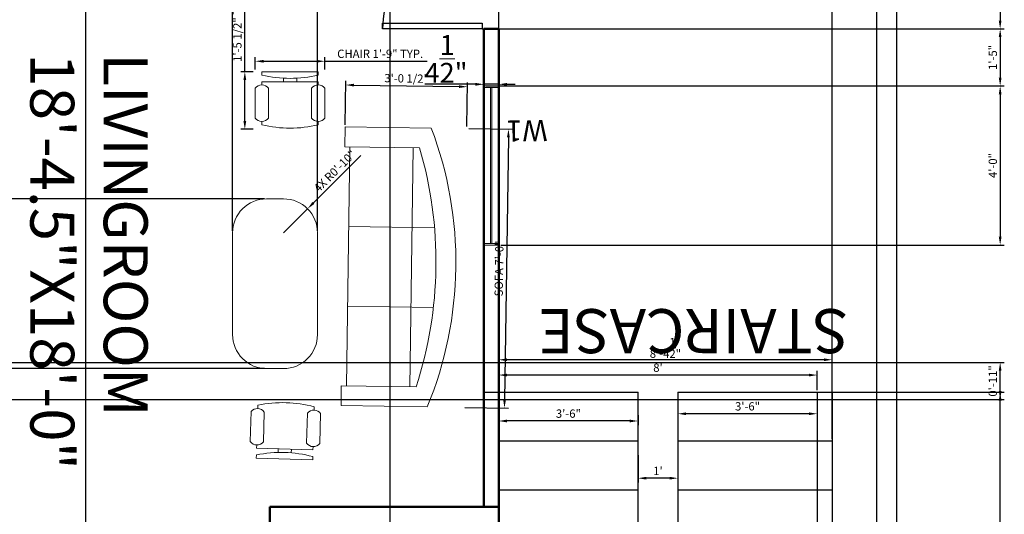
# Model space of a CAD drawing. Units: inches. Extents: x 1989 to 2637, y 1032 to 1611.
# Tile 4 of 5: x 2340 to 2637, y 1274 to 1423. Entities that reach past the tile are written whole.
import ezdxf

# ---------------------------------------------------------------- set-up
doc = ezdxf.new("R2010")
doc.units = ezdxf.units.IN
for name, color, linetype, lineweight in [('A-ANNO-TEXT', 1, 'Continuous', 18), ('A-AREA-IDEN', 1, 'Continuous', 25), ('C-PROP', 7, 'Continuous', 25), ('DIMENSIONS', 7, 'Continuous', 18), ('doors', 5, 'Continuous', 25), ('furniture', 8, 'Continuous', 18), ('stair case', 6, 'Continuous', 25), ('walls', 7, 'Continuous', 50), ('windows', 3, 'Continuous', 18)]:
    doc.layers.add(name, color=color, linetype=linetype, lineweight=lineweight)
doc.styles.get("Standard").update_dxf_attribs({"font": 'arial.ttf'})
doc.dimstyles.new('ISO-25', dxfattribs={"dimtxt": 2.5, "dimasz": 2.5, "dimexe": 1.25, "dimexo": 0.625, "dimtad": 1, "dimlunit": 4, "dimtxsty": 'Standard', "dimcen": 2.5, "dimadec": 0, "dimazin": 0, "dimtfac": 1, "dimtmove": 0, "dimatfit": 3, "dimfxl": 1, "dimarcsym": 0})

# ---------------------------------------------------------------- blocks, each defined once
blk = doc.blocks.new('*U2')
for p, q in [((0, 0), (0, -5)), ((30, 0), (30, -5))]:
    blk.add_line(p, q)
blk.add_lwpolyline([(0, 0), (0, 30), (1.75, 30), (1.75, 0)], close=True)
blk.add_arc((0, 0), 30, 0, 90)
blk = doc.blocks.new('Sofa - Roundback 7 ft.')
for p, q in [((-12.00002, -32.4421), (-12.00003, -6.5971)), ((11.99997, -32.4421), (11.99998, -6.5971)), ((-36.000027, -34), (-36.000027, -11.4696)), ((35.99998, -34), (35.99998, -11.4696)), ((-35.999844, -13.3819), (35.9998, -13.3819)), ((-36.000027, -32.4421), (35.99998, -32.4421))]:
    blk.add_line(p, q)
for points in [[(-36.000027, -34), (-42.000027, -34), (-42.000027, -8)], [(41.99998, -8), (41.99998, -34), (35.99998, -34)]]:
    blk.add_lwpolyline(points)
for centre, radius, start, end in [((0, -114.25), 114.25, 68.43141, 111.5686), ((-0.00001, -127.1968), 121.1968, 72.72033, 107.2797)]:
    blk.add_arc(centre, radius, start, end)
blk = doc.blocks.new('Chair - Desk')
for p, q in [((-8.5, 0), (-8.5, -1)), ((-8.5, 0), (8.5, 0)), ((8.5, 0), (8.5, -1)), ((-2, -3), (-2, -1.9355)), ((2, -1.9576), (2, -3)), ((-10.5, -5), (-10.5, -14)), ((-8.5, -3), (-8.5, -4)), ((-8.5, -3), (8.5, -3)), ((-6.5, -14), (-6.5, -5)), ((6.5, -5), (6.5, -14)), ((8.5, -3), (8.5, -4)), ((10.5, -14), (10.5, -5)), ((-8.5, -15), (-8.5, -16)), ((8.5, -15), (8.5, -16))]:
    blk.add_line(p, q)
for centre, radius, start, end in [((0, 34.625), 36.625, 256.5803, 283.4197), ((-8.5, -6.5), 2.5, 36.8699, 143.1301), ((8.5, -6.5), 2.5, 36.8699, 143.1301), ((-8.5, -12.5), 2.5, 216.8699, 323.1301), ((8.5, -12.5), 2.5, 216.8699, 323.1301), ((0, 19.625), 36.625, 256.5803, 283.4197)]:
    blk.add_arc(centre, radius, start, end)
blk = doc.blocks.new('*D13')
at = {"layer": 'Defpoints', "color": 0, "transparency": 16777216}
for p in [(2484.5, 1432.53), (2484.5, 1402.72), (2598.5, 1403.71)]:
    blk.add_point(p, dxfattribs=at)
at = {"layer": 'DIMENSIONS', "color": 0, "lineweight": -2, "transparency": 16777216}
for p, q in [((2484.5, 1403.34), (2484.5, 1433.78)), ((2598.5, 1404.33), (2598.5, 1433.78)), ((2596, 1432.53), (2487, 1432.53))]:
    blk.add_line(p, q, dxfattribs=at)
at = {"layer": 'DIMENSIONS', "color": 0, "transparency": 16777216}
for points in [[(2487, 1432.95), (2487, 1432.12), (2484.5, 1432.53)], [(2596, 1432.95), (2596, 1432.12), (2598.5, 1432.53)]]:
    blk.add_solid(points, dxfattribs=at)
at = {"layer": 'DIMENSIONS', "color": 0, "transparency": 16777216, "insert": (2541.5, 1436.22), "char_height": 6, "attachment_point": 5}
blk.add_mtext('9\'-6"', dxfattribs=at)
blk = doc.blocks.new('*D15')
at = {"layer": 'Defpoints', "color": 0, "transparency": 16777216}
for p in [(2480, 1411.38), (2484.5, 1411.38), (2480, 1403.71)]:
    blk.add_point(p, dxfattribs=at)
at = {"layer": 'DIMENSIONS', "color": 0, "lineweight": -2, "transparency": 16777216}
for p, q in [((2480, 1410.76), (2480, 1402.46)), ((2484.5, 1410.76), (2484.5, 1402.46)), ((2477.5, 1403.71), (2462.23, 1403.71)), ((2484.5, 1403.71), (2480, 1403.71)), ((2487, 1403.71), (2489.5, 1403.71))]:
    blk.add_line(p, q, dxfattribs=at)
at = {"layer": 'DIMENSIONS', "color": 0, "transparency": 16777216}
for points in [[(2477.5, 1404.13), (2477.5, 1403.3), (2480, 1403.71)], [(2487, 1404.13), (2487, 1403.3), (2484.5, 1403.71)]]:
    blk.add_solid(points, dxfattribs=at)
at = {"layer": 'DIMENSIONS', "color": 0, "transparency": 16777216, "insert": (2468.62, 1411.36), "char_height": 6, "attachment_point": 5}
blk.add_mtext('4{\\H1x;\\S1/2;}"', dxfattribs=at)
blk = doc.blocks.new('*D17')
at = {"layer": 'Defpoints', "color": 0, "transparency": 16777216}
for p in [(2538.5, 1310.92), (2580.5, 1310.92), (2538.5, 1304.46)]:
    blk.add_point(p, dxfattribs=at)
at = {"layer": 'DIMENSIONS', "color": 0, "lineweight": -2, "transparency": 16777216}
for p, q in [((2538.5, 1310.3), (2538.5, 1303.21)), ((2580.5, 1310.3), (2580.5, 1303.21)), ((2578, 1304.46), (2541, 1304.46))]:
    blk.add_line(p, q, dxfattribs=at)
at = {"layer": 'DIMENSIONS', "color": 0, "transparency": 16777216}
for points in [[(2541, 1304.88), (2541, 1304.05), (2538.5, 1304.46)], [(2578, 1304.88), (2578, 1304.05), (2580.5, 1304.46)]]:
    blk.add_solid(points, dxfattribs=at)
at = {"layer": 'DIMENSIONS', "color": 0, "transparency": 16777216, "insert": (2559.5, 1306.37), "char_height": 2.5, "attachment_point": 5}
blk.add_mtext('3\'-6"', dxfattribs=at)
blk = doc.blocks.new('*D18')
at = {"layer": 'Defpoints', "color": 0, "transparency": 16777216}
for p in [(2526.5, 1292.57), (2538.5, 1292.57), (2526.5, 1285.04)]:
    blk.add_point(p, dxfattribs=at)
at = {"layer": 'DIMENSIONS', "color": 0, "lineweight": -2, "transparency": 16777216}
for p, q in [((2526.5, 1291.94), (2526.5, 1283.79)), ((2538.5, 1291.94), (2538.5, 1283.79)), ((2536, 1285.04), (2529, 1285.04))]:
    blk.add_line(p, q, dxfattribs=at)
at = {"layer": 'DIMENSIONS', "color": 0, "transparency": 16777216}
for points in [[(2529, 1285.46), (2529, 1284.63), (2526.5, 1285.04)], [(2536, 1285.46), (2536, 1284.63), (2538.5, 1285.04)]]:
    blk.add_solid(points, dxfattribs=at)
at = {"layer": 'DIMENSIONS', "color": 0, "transparency": 16777216, "insert": (2532.5, 1286.92), "char_height": 2.5, "attachment_point": 5}
blk.add_mtext("1'", dxfattribs=at)
blk = doc.blocks.new('*D19')
at = {"layer": 'Defpoints', "color": 0, "transparency": 16777216}
for p in [(2484.5, 1304.71), (2526.5, 1304.71), (2484.5, 1302.28)]:
    blk.add_point(p, dxfattribs=at)
at = {"layer": 'DIMENSIONS', "color": 0, "lineweight": -2, "transparency": 16777216}
for p, q in [((2484.5, 1304.08), (2484.5, 1301.03)), ((2526.5, 1304.08), (2526.5, 1301.03)), ((2524, 1302.28), (2487, 1302.28))]:
    blk.add_line(p, q, dxfattribs=at)
at = {"layer": 'DIMENSIONS', "color": 0, "transparency": 16777216}
for points in [[(2487, 1302.7), (2487, 1301.86), (2484.5, 1302.28)], [(2524, 1302.7), (2524, 1301.86), (2526.5, 1302.28)]]:
    blk.add_solid(points, dxfattribs=at)
at = {"layer": 'DIMENSIONS', "color": 0, "transparency": 16777216, "insert": (2505.5, 1304.18), "char_height": 2.5, "attachment_point": 5}
blk.add_mtext('3\'-6"', dxfattribs=at)
blk = doc.blocks.new('*D20')
at = {"layer": 'Defpoints', "color": 0, "transparency": 16777216}
for p in [(2484.5, 1316.12), (2484.5, 1310.92), (2580.5, 1310.92)]:
    blk.add_point(p, dxfattribs=at)
at = {"layer": 'DIMENSIONS', "color": 0, "lineweight": -2, "transparency": 16777216}
for p, q in [((2484.5, 1311.55), (2484.5, 1317.37)), ((2578, 1316.12), (2487, 1316.12)), ((2580.5, 1311.55), (2580.5, 1317.37))]:
    blk.add_line(p, q, dxfattribs=at)
at = {"layer": 'DIMENSIONS', "color": 0, "transparency": 16777216}
for points in [[(2487, 1316.53), (2487, 1315.7), (2484.5, 1316.12)], [(2578, 1316.53), (2578, 1315.7), (2580.5, 1316.12)]]:
    blk.add_solid(points, dxfattribs=at)
at = {"layer": 'DIMENSIONS', "color": 0, "transparency": 16777216, "insert": (2532.5, 1318.02), "char_height": 2.5, "attachment_point": 5}
blk.add_mtext("8'", dxfattribs=at)
blk = doc.blocks.new('*D21')
at = {"layer": 'Defpoints', "color": 0, "transparency": 16777216}
for p in [(2484.5, 1320.73), (2484.5, 1296.25), (2585, 1296.25)]:
    blk.add_point(p, dxfattribs=at)
at = {"layer": 'DIMENSIONS', "color": 0, "lineweight": -2, "transparency": 16777216}
for p, q in [((2484.5, 1296.88), (2484.5, 1321.98)), ((2582.5, 1320.73), (2487, 1320.73)), ((2585, 1296.88), (2585, 1321.98))]:
    blk.add_line(p, q, dxfattribs=at)
at = {"layer": 'DIMENSIONS', "color": 0, "transparency": 16777216}
for points in [[(2487, 1321.15), (2487, 1320.31), (2484.5, 1320.73)], [(2582.5, 1321.15), (2582.5, 1320.31), (2585, 1320.73)]]:
    blk.add_solid(points, dxfattribs=at)
at = {"layer": 'DIMENSIONS', "color": 0, "transparency": 16777216, "insert": (2534.75, 1324.3), "char_height": 2.5, "attachment_point": 5}
blk.add_mtext('8\'-4{\\H1x;\\S1/2;}"', dxfattribs=at)
blk = doc.blocks.new('*D28')
at = {"layer": 'Defpoints', "color": 0, "transparency": 16777216}
for p in [(2432.12, 1410.66), (2411.12, 1407.51), (2432.12, 1407.51)]:
    blk.add_point(p, dxfattribs=at)
at = {"layer": 'DIMENSIONS', "color": 0, "lineweight": -2, "transparency": 16777216}
for p, q in [((2411.12, 1408.13), (2411.12, 1411.91)), ((2413.62, 1410.66), (2429.62, 1410.66)), ((2432.12, 1408.13), (2432.12, 1411.91)), ((2432.12, 1410.66), (2462.92, 1410.66))]:
    blk.add_line(p, q, dxfattribs=at)
at = {"layer": 'DIMENSIONS', "color": 0, "transparency": 16777216}
for points in [[(2413.62, 1411.07), (2413.62, 1410.24), (2411.12, 1410.66)], [(2429.62, 1411.07), (2429.62, 1410.24), (2432.12, 1410.66)]]:
    blk.add_solid(points, dxfattribs=at)
at = {"layer": 'DIMENSIONS', "color": 0, "transparency": 16777216, "insert": (2448.77, 1412.58), "char_height": 2.5, "attachment_point": 5}
blk.add_mtext('CHAIR 1\'-9" TYP.', dxfattribs=at)
blk = doc.blocks.new('*D29')
at = {"layer": 'Defpoints', "color": 0, "transparency": 16777216}
for p in [(2407.97, 1407.51), (2411.12, 1407.51), (2411.12, 1390.17)]:
    blk.add_point(p, dxfattribs=at)
at = {"layer": 'DIMENSIONS', "color": 0, "lineweight": -2, "transparency": 16777216}
for p, q in [((2407.97, 1407.51), (2407.97, 1432.09)), ((2410.49, 1407.51), (2406.72, 1407.51)), ((2407.97, 1392.67), (2407.97, 1405.01)), ((2410.49, 1390.17), (2406.72, 1390.17))]:
    blk.add_line(p, q, dxfattribs=at)
at = {"layer": 'DIMENSIONS', "color": 0, "transparency": 16777216}
for points in [[(2407.55, 1405.01), (2408.39, 1405.01), (2407.97, 1407.51)], [(2407.55, 1392.67), (2408.39, 1392.67), (2407.97, 1390.17)]]:
    blk.add_solid(points, dxfattribs=at)
at = {"layer": 'DIMENSIONS', "color": 0, "transparency": 16777216, "insert": (2406.05, 1421.05), "char_height": 2.5, "attachment_point": 5, "rotation": 90}
blk.add_mtext('1\'-5 1/2" TYP.', dxfattribs=at)
blk = doc.blocks.new('*D36')
at = {"layer": 'Defpoints', "color": 0, "transparency": 16777216}
for p in [(2474.85, 1390.38), (2473.63, 1306.39), (2486.23, 1306.2)]:
    blk.add_point(p, dxfattribs=at)
at = {"layer": 'DIMENSIONS', "color": 0, "lineweight": -2, "transparency": 16777216}
for p, q in [((2475.47, 1390.37), (2488.7, 1390.18)), ((2487.41, 1387.7), (2486.27, 1308.7)), ((2474.26, 1306.38), (2487.48, 1306.19))]:
    blk.add_line(p, q, dxfattribs=at)
at = {"layer": 'DIMENSIONS', "color": 0, "transparency": 16777216}
for points in [[(2486.99, 1387.7), (2487.83, 1387.69), (2487.45, 1390.2)], [(2485.85, 1308.71), (2486.68, 1308.7), (2486.23, 1306.2)]]:
    blk.add_solid(points, dxfattribs=at)
at = {"layer": 'DIMENSIONS', "color": 0, "transparency": 16777216, "insert": (2484.92, 1348.23), "char_height": 2.5, "attachment_point": 5, "rotation": 89.1706}
blk.add_mtext('SOFA 7\'-0"', dxfattribs=at)
blk = doc.blocks.new('*D37')
at = {"layer": 'Defpoints', "color": 0, "transparency": 16777216}
for p in [(2475.03, 1402.98), (2438.19, 1390.91), (2474.85, 1390.38)]:
    blk.add_point(p, dxfattribs=at)
at = {"layer": 'DIMENSIONS', "color": 0, "lineweight": -2, "transparency": 16777216}
for p, q in [((2438.2, 1391.53), (2438.39, 1404.76)), ((2474.86, 1391), (2475.05, 1404.23)), ((2440.87, 1403.47), (2472.53, 1403.01))]:
    blk.add_line(p, q, dxfattribs=at)
at = {"layer": 'DIMENSIONS', "color": 0, "transparency": 16777216}
for points in [[(2440.87, 1403.89), (2440.86, 1403.05), (2438.37, 1403.51)], [(2472.54, 1403.43), (2472.53, 1402.6), (2475.03, 1402.98)]]:
    blk.add_solid(points, dxfattribs=at)
at = {"layer": 'DIMENSIONS', "color": 0, "transparency": 16777216, "insert": (2456.73, 1405.16), "char_height": 2.5, "attachment_point": 5, "rotation": 359.1706}
blk.add_mtext('3\'-0 1/2"', dxfattribs=at)
blk = doc.blocks.new('*D40')
at = {"layer": 'Defpoints', "color": 0, "transparency": 16777216}
for p in [(2585, 1576.07), (2082.5, 1496.92), (2585, 1310.92)]:
    blk.add_point(p, dxfattribs=at)
at = {"layer": 'DIMENSIONS', "color": 0, "lineweight": -2, "transparency": 16777216}
for p, q in [((2082.5, 1497.55), (2082.5, 1577.32)), ((2085, 1576.07), (2582.5, 1576.07)), ((2585, 1311.55), (2585, 1577.32))]:
    blk.add_line(p, q, dxfattribs=at)
at = {"layer": 'DIMENSIONS', "color": 0, "transparency": 16777216}
for points in [[(2085, 1576.49), (2085, 1575.65), (2082.5, 1576.07)], [(2582.5, 1576.49), (2582.5, 1575.65), (2585, 1576.07)]]:
    blk.add_solid(points, dxfattribs=at)
at = {"layer": 'DIMENSIONS', "color": 0, "transparency": 16777216, "insert": (2333.75, 1577.99), "char_height": 2.5, "attachment_point": 5}
blk.add_mtext('41\'-10 1/2"', dxfattribs=at)
blk = doc.blocks.new('*D42')
at = {"layer": 'Defpoints', "color": 0, "transparency": 16777216}
for p in [(2484.5, 1480.42), (2484.5, 1420.42), (2635.65, 1420.42)]:
    blk.add_point(p, dxfattribs=at)
at = {"layer": 'DIMENSIONS', "color": 0, "lineweight": -2, "transparency": 16777216}
for p, q in [((2485.12, 1480.42), (2636.9, 1480.42)), ((2635.65, 1477.92), (2635.65, 1422.92)), ((2485.12, 1420.42), (2636.9, 1420.42))]:
    blk.add_line(p, q, dxfattribs=at)
at = {"layer": 'DIMENSIONS', "color": 0, "transparency": 16777216}
for points in [[(2635.23, 1477.92), (2636.06, 1477.92), (2635.65, 1480.42)], [(2635.23, 1422.92), (2636.06, 1422.92), (2635.65, 1420.42)]]:
    blk.add_solid(points, dxfattribs=at)
at = {"layer": 'DIMENSIONS', "color": 0, "transparency": 16777216, "insert": (2633.75, 1450.42), "char_height": 2.5, "attachment_point": 5, "rotation": 90}
blk.add_mtext('5\'-0"', dxfattribs=at)
blk = doc.blocks.new('*D46')
at = {"layer": 'Defpoints', "color": 0, "transparency": 16777216}
for p in [(2484.5, 1403.22), (2484.5, 1355.27), (2635.65, 1355.27)]:
    blk.add_point(p, dxfattribs=at)
at = {"layer": 'DIMENSIONS', "color": 0, "lineweight": -2, "transparency": 16777216}
for p, q in [((2485.12, 1403.22), (2636.9, 1403.22)), ((2635.65, 1400.72), (2635.65, 1357.77)), ((2485.12, 1355.27), (2636.9, 1355.27))]:
    blk.add_line(p, q, dxfattribs=at)
at = {"layer": 'DIMENSIONS', "color": 0, "transparency": 16777216}
for points in [[(2635.23, 1400.72), (2636.06, 1400.72), (2635.65, 1403.22)], [(2635.23, 1357.77), (2636.06, 1357.77), (2635.65, 1355.27)]]:
    blk.add_solid(points, dxfattribs=at)
at = {"layer": 'DIMENSIONS', "color": 0, "transparency": 16777216, "insert": (2633.75, 1379.24), "char_height": 2.5, "attachment_point": 5, "rotation": 90}
blk.add_mtext('4\'-0"', dxfattribs=at)
blk = doc.blocks.new('*D47')
at = {"layer": 'Defpoints', "color": 0, "transparency": 16777216}
for p in [(2580.5, 1310.92), (2635.65, 1310.92), (2585, 1178.92)]:
    blk.add_point(p, dxfattribs=at)
at = {"layer": 'DIMENSIONS', "color": 0, "lineweight": -2, "transparency": 16777216}
for p, q in [((2581.12, 1310.92), (2636.9, 1310.92)), ((2635.65, 1181.42), (2635.65, 1308.42)), ((2585.62, 1178.92), (2636.9, 1178.92))]:
    blk.add_line(p, q, dxfattribs=at)
at = {"layer": 'DIMENSIONS', "color": 0, "transparency": 16777216}
for points in [[(2635.23, 1308.42), (2636.06, 1308.42), (2635.65, 1310.92)], [(2635.23, 1181.42), (2636.06, 1181.42), (2635.65, 1178.92)]]:
    blk.add_solid(points, dxfattribs=at)
at = {"layer": 'DIMENSIONS', "color": 0, "transparency": 16777216, "insert": (2633.75, 1244.92), "char_height": 2.5, "attachment_point": 5, "rotation": 90}
blk.add_mtext('11\'-0"', dxfattribs=at)
blk = doc.blocks.new('*D54')
at = {"layer": 'Defpoints', "color": 0, "transparency": 16777216}
for p in [(2429.87, 1576.07), (2404.3, 1358.98), (2429.87, 1358.98)]:
    blk.add_point(p, dxfattribs=at)
at = {"layer": 'DIMENSIONS', "color": 0, "lineweight": -2, "transparency": 16777216}
for p, q in [((2404.3, 1359.6), (2404.3, 1577.32)), ((2406.8, 1576.07), (2427.37, 1576.07)), ((2429.87, 1359.6), (2429.87, 1577.32))]:
    blk.add_line(p, q, dxfattribs=at)
at = {"layer": 'DIMENSIONS', "color": 0, "transparency": 16777216}
for points in [[(2406.8, 1576.49), (2406.8, 1575.65), (2404.3, 1576.07)], [(2427.37, 1576.49), (2427.37, 1575.65), (2429.87, 1576.07)]]:
    blk.add_solid(points, dxfattribs=at)
at = {"layer": 'DIMENSIONS', "color": 0, "transparency": 16777216, "insert": (2417.08, 1577.99), "char_height": 2.5, "attachment_point": 5}
blk.add_mtext('2\'-1 1/2"', dxfattribs=at)
blk = doc.blocks.new('*D55')
at = {"layer": 'Defpoints', "color": 0, "transparency": 16777216}
for p in [(2414.53, 1369.21), (2033.35, 1318.07), (2414.53, 1318.07)]:
    blk.add_point(p, dxfattribs=at)
at = {"layer": 'DIMENSIONS', "color": 0, "lineweight": -2, "transparency": 16777216}
for p, q in [((2413.9, 1369.21), (2032.1, 1369.21)), ((2033.35, 1366.71), (2033.35, 1320.57)), ((2413.9, 1318.07), (2032.1, 1318.07))]:
    blk.add_line(p, q, dxfattribs=at)
at = {"layer": 'DIMENSIONS', "color": 0, "transparency": 16777216}
for points in [[(2032.93, 1366.71), (2033.76, 1366.71), (2033.35, 1369.21)], [(2032.93, 1320.57), (2033.76, 1320.57), (2033.35, 1318.07)]]:
    blk.add_solid(points, dxfattribs=at)
at = {"layer": 'DIMENSIONS', "color": 0, "transparency": 16777216, "insert": (2031.45, 1343.64), "char_height": 2.5, "attachment_point": 5, "rotation": 90}
blk.add_mtext('4\'-3"', dxfattribs=at)
blk = doc.blocks.new('*D58')
at = {"layer": 'Defpoints', "color": 0, "transparency": 16777216}
for p in [(2480, 1420.42), (2480, 1403.22), (2635.65, 1403.22)]:
    blk.add_point(p, dxfattribs=at)
at = {"layer": 'DIMENSIONS', "color": 0, "lineweight": -2, "transparency": 16777216}
for p, q in [((2480.62, 1420.42), (2636.9, 1420.42)), ((2635.65, 1417.92), (2635.65, 1405.72)), ((2480.62, 1403.22), (2636.9, 1403.22))]:
    blk.add_line(p, q, dxfattribs=at)
at = {"layer": 'DIMENSIONS', "color": 0, "transparency": 16777216}
for points in [[(2635.23, 1417.92), (2636.06, 1417.92), (2635.65, 1420.42)], [(2635.23, 1405.72), (2636.06, 1405.72), (2635.65, 1403.22)]]:
    blk.add_solid(points, dxfattribs=at)
at = {"layer": 'DIMENSIONS', "color": 0, "transparency": 16777216, "insert": (2633.75, 1411.82), "char_height": 2.5, "attachment_point": 5, "rotation": 90}
blk.add_mtext('1\'-5"', dxfattribs=at)
blk = doc.blocks.new('*D60')
at = {"layer": 'Defpoints', "color": 0, "transparency": 16777216}
for p in [(2451.78, 1576.07), (2360, 1087.42), (2451.78, 1087.42)]:
    blk.add_point(p, dxfattribs=at)
at = {"layer": 'DIMENSIONS', "color": 0, "lineweight": -2, "transparency": 16777216}
for p, q in [((2360, 1088.05), (2360, 1577.32)), ((2362.5, 1576.07), (2449.28, 1576.07)), ((2451.78, 1088.05), (2451.78, 1577.32))]:
    blk.add_line(p, q, dxfattribs=at)
at = {"layer": 'DIMENSIONS', "color": 0, "transparency": 16777216}
for points in [[(2362.5, 1576.49), (2362.5, 1575.65), (2360, 1576.07)], [(2449.28, 1576.49), (2449.28, 1575.65), (2451.78, 1576.07)]]:
    blk.add_solid(points, dxfattribs=at)
at = {"layer": 'DIMENSIONS', "color": 0, "transparency": 16777216, "insert": (2405.89, 1577.97), "char_height": 2.5, "attachment_point": 5}
blk.add_mtext('7\'-8"', dxfattribs=at)
blk = doc.blocks.new('*D63')
at = {"layer": 'Defpoints', "color": 0, "transparency": 16777216}
for p in [(2087, 1319.92), (2635.65, 1319.92), (2087, 1308.78)]:
    blk.add_point(p, dxfattribs=at)
at = {"layer": 'DIMENSIONS', "color": 0, "lineweight": -2, "transparency": 16777216}
for p, q in [((2087.62, 1319.92), (2636.9, 1319.92)), ((2635.65, 1311.28), (2635.65, 1317.42)), ((2087.62, 1308.78), (2636.9, 1308.78))]:
    blk.add_line(p, q, dxfattribs=at)
at = {"layer": 'DIMENSIONS', "color": 0, "transparency": 16777216}
for points in [[(2635.23, 1317.42), (2636.06, 1317.42), (2635.65, 1319.92)], [(2635.23, 1311.28), (2636.06, 1311.28), (2635.65, 1308.78)]]:
    blk.add_solid(points, dxfattribs=at)
at = {"layer": 'DIMENSIONS', "color": 0, "transparency": 16777216, "insert": (2633.75, 1314.35), "char_height": 2.5, "attachment_point": 5, "rotation": 90}
blk.add_mtext('0\'-11"', dxfattribs=at)
blk = doc.blocks.new('*D66')
at = {"layer": 'Defpoints', "color": 0, "transparency": 16777216}
for p in [(2426.87, 1366.21), (2419.64, 1358.98)]:
    blk.add_point(p, dxfattribs=at)
at = {"layer": 'DIMENSIONS', "color": 0, "lineweight": -2, "transparency": 16777216}
for p, q in [((2442.93, 1382.27), (2428.64, 1367.98)), ((2419.64, 1358.98), (2426.87, 1366.21))]:
    blk.add_line(p, q, dxfattribs=at)
at = {"layer": 'DIMENSIONS', "color": 0, "transparency": 16777216}
blk.add_solid([(2428.35, 1368.27), (2428.94, 1367.68), (2426.87, 1366.21)], dxfattribs=at)
at = {"layer": 'DIMENSIONS', "color": 0, "transparency": 16777216, "insert": (2435.32, 1377.35), "char_height": 2.5, "attachment_point": 5, "rotation": 45.002}
blk.add_mtext('4X R0\'-10"', dxfattribs=at)

msp = doc.modelspace()

# ---------------------------------------------------------------- linework, layer by layer
at = {"layer": 'C-PROP'}
for p, q in [((2604.498, 1064.921), (2604.498, 1544.921)), ((2598.498, 1070.921), (2598.498, 1538.921))]:
    msp.add_line(p, q, dxfattribs=at)
at = {"layer": 'furniture'}
msp.add_lwpolyline([(2429.87, 1358.979, 0.4142136), (2419.641, 1369.207), (2414.527, 1369.207, 0.4142136), (2404.299, 1358.979), (2404.299, 1328.294, 0.4142136), (2414.527, 1318.065), (2419.641, 1318.065, 0.4142136), (2429.87, 1328.294)], format="xyb", close=True, dxfattribs=at)
at = {"layer": 'stair case'}
for p, q in [((2479.998, 1310.921), (2526.498, 1310.921)), ((2479.998, 1310.921), (2526.498, 1310.921)), ((2484.498, 1070.921), (2484.498, 1310.921)), ((2526.498, 1178.921), (2526.498, 1310.921)), ((2538.498, 1310.921), (2538.498, 1178.921)), ((2538.498, 1310.921), (2584.998, 1310.921)), ((2538.498, 1310.921), (2584.998, 1310.921)), ((2580.498, 1310.921), (2580.498, 1070.921)), ((2584.998, 1310.921), (2584.998, 1070.921)), ((2484.498, 1296.254), (2526.498, 1296.254)), ((2538.498, 1296.254), (2584.998, 1296.254)), ((2484.498, 1281.588), (2526.498, 1281.588)), ((2538.498, 1281.588), (2584.998, 1281.588))]:
    msp.add_line(p, q, dxfattribs=at)
at = {"layer": 'walls'}
for p, q in [((2479.998, 1420.421), (2479.998, 1276.421)), ((2479.998, 1420.421), (2484.498, 1420.421)), ((2484.498, 1420.421), (2484.498, 1276.421)), ((2484.498, 1310.921), (2484.498, 1070.921)), ((2415.498, 1276.421), (2484.498, 1276.421)), ((2415.498, 1276.421), (2415.498, 1259.921))]:
    msp.add_line(p, q, dxfattribs=at)
at = {"layer": 'windows'}
for p, q in [((2479.998, 1355.269), (2479.998, 1403.219)), ((2479.998, 1403.219), (2484.498, 1403.219)), ((2479.998, 1402.719), (2484.498, 1402.719)), ((2482.048, 1402.719), (2482.048, 1355.769)), ((2482.448, 1402.719), (2482.448, 1355.769)), ((2484.498, 1403.219), (2484.498, 1355.269)), ((2484.498, 1355.769), (2479.998, 1355.769)), ((2484.498, 1355.269), (2479.998, 1355.269))]:
    msp.add_line(p, q, dxfattribs=at)

# ---------------------------------------------------------------- block references
at = {"layer": 'doors', "rotation": 89.99999999999999}
msp.add_blockref('*U2', (2479.498, 1420.421), dxfattribs=at)
at = {"layer": 'furniture'}
msp.add_blockref('Chair - Desk', (2421.619, 1407.508), dxfattribs=at)
at = {"layer": 'furniture', "rotation": 269.1705843501265}
msp.add_blockref('Sofa - Roundback 7 ft.', (2471.575, 1348.421), dxfattribs=at)
at = {"layer": 'furniture', "xscale": -1, "rotation": 178.3411687002522}
msp.add_blockref('Chair - Desk', (2419.929, 1290.805), dxfattribs=at)

# ---------------------------------------------------------------- texts
at = {"layer": 'A-ANNO-TEXT', "insert": (2499.262, 1386.594), "char_height": 6.3507, "attachment_point": 1, "rotation": 180.67334}
msp.add_mtext_dynamic_manual_height_columns('W1', width=5.29651, gutter_width=31.753, heights=[0], dxfattribs=at)
at = {"layer": 'A-AREA-IDEN', "attachment_point": 1}
for s, insert, char_height, rotation in [('LIVINGROOM\\P18\'-4.5"X18\'-0"', (2378.703, 1413.037), 13.26964, 270), ('STAIRCASE', (2589.929, 1322.707), 13.2696, 180)]:
    msp.add_mtext_dynamic_manual_height_columns(s, width=13.72319, gutter_width=66.348, heights=[0], dxfattribs=dict(at, insert=insert, char_height=char_height, rotation=rotation))

# ---------------------------------------------------------------- dimensions: what is measured, and where the dimension line sits
at = {"layer": 'DIMENSIONS'}
for base, p1, p2, override, picture, middle in [((2584.998, 1576.071), (2082.498, 1496.921), (2584.998, 1310.921), {"dimdec": 1, "dimlfac": 1, "dimrnd": 0, "dimzin": 1, "dimdsep": 46, "dimlunit": 4, "dimfrac": 2}, '*D40', (2333.748, 1577.989)), ((2451.776, 1576.071), (2359.998, 1087.421), (2451.776, 1087.421), {"dimdec": 1, "dimlfac": 1, "dimrnd": 0, "dimzin": 1, "dimdsep": 46, "dimlunit": 4, "dimfrac": 2}, '*D60', (2405.887, 1577.972)), ((2429.87, 1576.071), (2404.299, 1358.979), (2429.87, 1358.979), {"dimdec": 1, "dimlfac": 1, "dimrnd": 0, "dimzin": 1, "dimdsep": 46, "dimlunit": 4, "dimfrac": 2}, '*D54', (2417.084, 1577.989)), ((2484.498, 1432.534), (2598.498, 1403.705), (2484.498, 1402.719), {"dimtxt": 6, "dimclrd": 0, "dimclre": 0, "dimclrt": 0}, '*D13', (2541.498, 1436.223)), ((2479.998, 1403.714), (2484.498, 1411.384), (2479.998, 1411.384), {"dimtxt": 6, "dimclrd": 0, "dimclre": 0, "dimclrt": 0}, '*D15', (2468.616, 1411.363)), ((2484.498, 1320.729), (2584.998, 1296.254), (2484.498, 1296.254), {"dimclrd": 0, "dimclre": 0, "dimclrt": 0}, '*D21', (2534.748, 1324.302)), ((2484.498, 1316.117), (2580.498, 1310.921), (2484.498, 1310.921), {"dimclrd": 0, "dimclre": 0, "dimclrt": 0}, '*D20', (2532.498, 1318.018)), ((2538.498, 1304.465), (2580.498, 1310.921), (2538.498, 1310.921), {"dimclrd": 0, "dimclre": 0, "dimclrt": 0}, '*D17', (2559.498, 1306.367)), ((2484.498, 1302.28), (2526.498, 1304.707), (2484.498, 1304.707), {"dimclrd": 0, "dimclre": 0, "dimclrt": 0}, '*D19', (2505.498, 1304.182)), ((2526.498, 1285.044), (2538.498, 1292.57), (2526.498, 1292.57), {"dimclrd": 0, "dimclre": 0, "dimclrt": 0}, '*D18', (2532.498, 1286.925))]:
    dim = msp.add_linear_dim(base=base, p1=p1, p2=p2, dimstyle='ISO-25', override=override, dxfattribs=at)
    dim.commit()
    dim.dimension.update_dxf_attribs({"geometry": picture, "text_midpoint": middle})
for base, p1, p2, angle, picture, middle in [((2635.648, 1420.421), (2484.498, 1480.421), (2484.498, 1420.421), 90, '*D42', (2633.746, 1450.421)), ((2635.648, 1403.219), (2479.998, 1420.421), (2479.998, 1403.219), 90, '*D58', (2633.746, 1411.82)), ((2475.031, 1402.977), (2438.186, 1390.909), (2474.849, 1390.378), 359.17058, '*D37', (2456.728, 1405.16)), ((2635.6477, 1355.2692), (2484.4977, 1403.2189), (2484.4977, 1355.2692), 90, '*D46', (2633.7463, 1379.244)), ((2033.348, 1318.065), (2414.527, 1369.207), (2414.527, 1318.065), 90, '*D55', (2031.445, 1343.636)), ((2635.648, 1319.921), (2086.998, 1308.778), (2086.998, 1319.921), 90, '*D63', (2633.746, 1314.349)), ((2635.648, 1310.921), (2584.998, 1178.921), (2580.498, 1310.921), 90, '*D47', (2633.746, 1244.921))]:
    dim = msp.add_linear_dim(base=base, p1=p1, p2=p2, angle=angle, dimstyle='ISO-25', override={"dimdec": 1, "dimlfac": 1, "dimrnd": 0, "dimzin": 1, "dimdsep": 46, "dimlunit": 4, "dimfrac": 2}, dxfattribs=at)
    dim.commit()
    dim.dimension.update_dxf_attribs({"geometry": picture, "text_midpoint": middle})
for base, p1, p2, angle, text, picture, middle in [((2407.969, 1407.508), (2411.119, 1390.175), (2411.119, 1407.508), 90, '<> TYP.', '*D29', (2406.051, 1421.047)), ((2486.232, 1306.204), (2474.849, 1390.378), (2473.633, 1306.387), 269.17058, 'SOFA <>', '*D36', (2484.921, 1348.228))]:
    dim = msp.add_linear_dim(base=base, p1=p1, p2=p2, angle=angle, text=text, dimstyle='ISO-25', override={"dimdec": 1, "dimlfac": 1, "dimrnd": 0, "dimzin": 1, "dimdsep": 46, "dimlunit": 4, "dimfrac": 2}, dxfattribs=at)
    dim.commit()
    dim.dimension.update_dxf_attribs({"geometry": picture, "text_midpoint": middle})
dim = msp.add_linear_dim(base=(2432.119, 1410.658), p1=(2411.119, 1407.508), p2=(2432.119, 1407.508), text='CHAIR <> TYP.', dimstyle='ISO-25', override={"dimdec": 1, "dimlfac": 1, "dimrnd": 0, "dimzin": 1, "dimdsep": 46, "dimlunit": 4, "dimfrac": 2}, dxfattribs=at)
dim.commit()
dim.dimension.update_dxf_attribs({"geometry": '*D28', "text_midpoint": (2448.767, 1412.576)})
dim = msp.add_radius_dim(center=(2419.641, 1358.979), mpoint=(2426.874, 1366.212), text='4X <>', dimstyle='ISO-25', override={"dimdec": 1, "dimlfac": 1, "dimrnd": 0, "dimzin": 1, "dimdsep": 46, "dimlunit": 4, "dimfrac": 2}, dxfattribs=at)
dim.commit()
dim.dimension.update_dxf_attribs({"geometry": '*D66', "text_midpoint": (2435.323, 1377.351)})

doc.saveas('drawing.dxf')
